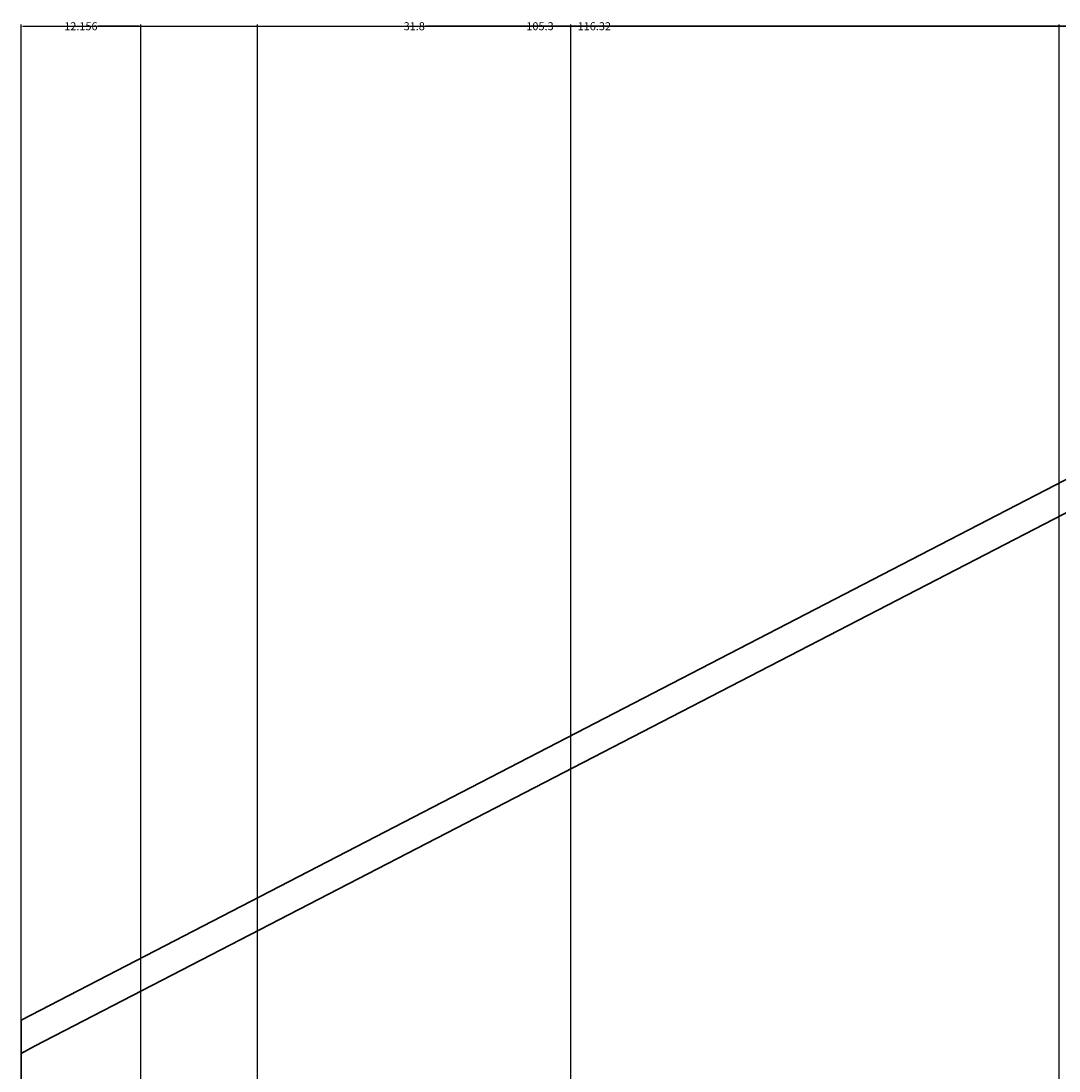
# Model space of a CAD drawing. Units: inches. Extents: x 69 to 650, y -16 to 573.
# Tile 16 of 26: x 100 to 205, y 466 to 573. Entities that reach past the tile are written whole.
import ezdxf

# ---------------------------------------------------------------- set-up
doc = ezdxf.new("R2010")
doc.units = ezdxf.units.IN
doc.header["$MEASUREMENT"] = 0
for name, color, linetype, lineweight in [('A-ANNO-DIMS', 2, 'Continuous', 18), ('A-ROOF', 7, 'Continuous', 35), ('A-WALL', 7, 'Continuous', 35)]:
    doc.layers.add(name, color=color, linetype=linetype, lineweight=lineweight)
doc.styles.get("Standard").update_dxf_attribs({"font": 'arial.ttf'})
doc.dimstyles.get("Standard").update_dxf_attribs({"dimtxt": 0.8125, "dimasz": 0.18, "dimexe": 0.18, "dimexo": 0.0625, "dimgap": 0.09, "dimtad": 0, "dimtih": 1, "dimtoh": 1, "dimdec": 4, "dimzin": 0, "dimdsep": 46, "dimlunit": 4, "dimtxsty": 'Standard', "dimcen": 0.09, "dimadec": 0, "dimazin": 0, "dimtfac": 1, "dimtdec": 4, "dimtofl": 0, "dimtmove": 0, "dimatfit": 3, "dimfxl": 1, "dimtolj": 1, "dimtzin": 0, "dimarcsym": 0})

# ---------------------------------------------------------------- blocks, each defined once
blk = doc.blocks.new('*D19')
at = {"layer": 'A-ANNO-DIMS', "color": 0, "lineweight": -2, "transparency": 16777216}
for p, q in [((99.56, 471.72), (99.56, 572.74)), ((99.74, 572.56), (358.57, 572.56)), ((619.38, 572.56), (360.54, 572.56)), ((619.56, 87.99), (619.56, 572.74))]:
    blk.add_line(p, q, dxfattribs=at)
at = {"layer": 'A-ANNO-DIMS', "color": 0, "transparency": 16777216}
for points in [[(99.74, 572.59), (99.74, 572.53), (99.56, 572.56)], [(619.38, 572.59), (619.38, 572.53), (619.56, 572.56)]]:
    blk.add_solid(points, dxfattribs=at)
at = {"layer": 'Defpoints', "color": 0, "transparency": 16777216}
for p in [(619.56, 572.56), (99.56, 471.66), (619.56, 87.93)]:
    blk.add_point(p, dxfattribs=at)
at = {"layer": 'A-ANNO-DIMS', "color": 0, "transparency": 16777216, "insert": (359.56, 572.56), "char_height": 0.812, "attachment_point": 5}
blk.add_mtext('\\A1;520', dxfattribs=at)
blk = doc.blocks.new('*D49')
at = {"layer": 'A-ANNO-DIMS', "color": 0, "lineweight": -2, "transparency": 16777216}
for p, q in [((99.56, 471.72), (99.56, 572.74)), ((99.74, 572.56), (155.98, 572.56)), ((215.7, 572.56), (159.45, 572.56)), ((215.88, 544.22), (215.88, 572.74))]:
    blk.add_line(p, q, dxfattribs=at)
at = {"layer": 'A-ANNO-DIMS', "color": 0, "transparency": 16777216}
for points in [[(99.74, 572.59), (99.74, 572.53), (99.56, 572.56)], [(215.7, 572.59), (215.7, 572.53), (215.88, 572.56)]]:
    blk.add_solid(points, dxfattribs=at)
at = {"layer": 'Defpoints', "color": 0, "transparency": 16777216}
for p in [(215.88, 572.56), (215.88, 544.16), (99.56, 471.66)]:
    blk.add_point(p, dxfattribs=at)
at = {"layer": 'A-ANNO-DIMS', "color": 0, "transparency": 16777216, "insert": (157.72, 572.56), "char_height": 0.812, "attachment_point": 5}
blk.add_mtext('\\A1;116.32', dxfattribs=at)
blk = doc.blocks.new('*D53')
at = {"layer": 'A-ANNO-DIMS', "color": 0, "lineweight": -2, "transparency": 16777216}
for p, q in [((99.56, 411.99), (99.56, 572.74)), ((99.74, 572.56), (103.9, 572.56)), ((111.53, 572.56), (107.37, 572.56)), ((111.71, 414.48), (111.71, 572.74))]:
    blk.add_line(p, q, dxfattribs=at)
at = {"layer": 'A-ANNO-DIMS', "color": 0, "transparency": 16777216}
for points in [[(99.74, 572.59), (99.74, 572.53), (99.56, 572.56)], [(111.53, 572.59), (111.53, 572.53), (111.71, 572.56)]]:
    blk.add_solid(points, dxfattribs=at)
at = {"layer": 'Defpoints', "color": 0, "transparency": 16777216}
for p in [(111.71, 572.56), (111.71, 414.41), (99.56, 411.93)]:
    blk.add_point(p, dxfattribs=at)
at = {"layer": 'A-ANNO-DIMS', "color": 0, "transparency": 16777216, "insert": (105.63, 572.56), "char_height": 0.812, "attachment_point": 5}
blk.add_mtext('\\A1;12.156', dxfattribs=at)
blk = doc.blocks.new('*D54')
at = {"layer": 'A-ANNO-DIMS', "color": 0, "lineweight": -2, "transparency": 16777216}
for p, q in [((123.55, 432.36), (123.55, 572.74)), ((123.73, 572.56), (138.31, 572.56)), ((155.17, 572.56), (140.6, 572.56)), ((155.35, 432.36), (155.35, 572.74))]:
    blk.add_line(p, q, dxfattribs=at)
at = {"layer": 'A-ANNO-DIMS', "color": 0, "transparency": 16777216}
for points in [[(123.73, 572.59), (123.73, 572.53), (123.55, 572.56)], [(155.17, 572.59), (155.17, 572.53), (155.35, 572.56)]]:
    blk.add_solid(points, dxfattribs=at)
at = {"layer": 'Defpoints', "color": 0, "transparency": 16777216}
for p in [(155.35, 572.56), (123.55, 432.3), (155.35, 432.3)]:
    blk.add_point(p, dxfattribs=at)
at = {"layer": 'A-ANNO-DIMS', "color": 0, "transparency": 16777216, "insert": (139.45, 572.56), "char_height": 0.812, "attachment_point": 5}
blk.add_mtext('\\A1;31.8', dxfattribs=at)
blk = doc.blocks.new('*D61')
at = {"layer": 'A-ANNO-DIMS', "color": 0, "lineweight": -2, "transparency": 16777216}
for p, q in [((99.56, 471.72), (99.56, 572.74)), ((99.74, 572.56), (150.79, 572.56)), ((204.69, 572.56), (153.63, 572.56)), ((204.87, 452.8), (204.87, 572.74))]:
    blk.add_line(p, q, dxfattribs=at)
at = {"layer": 'A-ANNO-DIMS', "color": 0, "transparency": 16777216}
for points in [[(99.74, 572.59), (99.74, 572.53), (99.56, 572.56)], [(204.69, 572.59), (204.69, 572.53), (204.87, 572.56)]]:
    blk.add_solid(points, dxfattribs=at)
at = {"layer": 'Defpoints', "color": 0, "transparency": 16777216}
for p in [(204.87, 572.56), (99.56, 471.66), (204.87, 452.74)]:
    blk.add_point(p, dxfattribs=at)
at = {"layer": 'A-ANNO-DIMS', "color": 0, "transparency": 16777216, "insert": (152.21, 572.56), "char_height": 0.812, "attachment_point": 5}
blk.add_mtext('\\A1;105.3', dxfattribs=at)
blk = doc.blocks.new('*D62')
at = {"layer": 'A-ANNO-DIMS', "color": 0, "lineweight": -2, "transparency": 16777216}
for p, q in [((204.87, 452.8), (204.87, 572.74)), ((205.05, 572.56), (356.52, 572.56)), ((510.91, 572.56), (359.44, 572.56)), ((511.09, 451.98), (511.09, 572.74))]:
    blk.add_line(p, q, dxfattribs=at)
at = {"layer": 'A-ANNO-DIMS', "color": 0, "transparency": 16777216}
for points in [[(205.05, 572.59), (205.05, 572.53), (204.87, 572.56)], [(510.91, 572.59), (510.91, 572.53), (511.09, 572.56)]]:
    blk.add_solid(points, dxfattribs=at)
at = {"layer": 'Defpoints', "color": 0, "transparency": 16777216}
for p in [(511.09, 572.56), (204.87, 452.74), (511.09, 451.92)]:
    blk.add_point(p, dxfattribs=at)
at = {"layer": 'A-ANNO-DIMS', "color": 0, "transparency": 16777216, "insert": (357.98, 572.56), "char_height": 0.812, "attachment_point": 5}
blk.add_mtext('\\A1;306.2', dxfattribs=at)

msp = doc.modelspace()

# ---------------------------------------------------------------- linework, layer by layer
at = {"layer": 'A-ROOF'}
for p, q in [((99.556, 471.6595), (218.848, 533.4142)), ((100.9352, 468.9953), (218.848, 530.036)), ((100.9352, 468.9953), (99.556, 468.2814))]:
    msp.add_line(p, q, dxfattribs=at)
at = {"layer": 'A-WALL'}
msp.add_line((99.556, 411.93), (99.556, 471.6595), dxfattribs=at)

# ---------------------------------------------------------------- dimensions: what is measured, and where the dimension line sits
at = {"layer": 'A-ANNO-DIMS'}
for base, p1, p2, override, picture, middle in [((619.555, 572.5573), (99.556, 471.6595), (619.555, 87.93), {"dimdec": 0, "dimlfac": 1, "dimrnd": 0, "dimzin": 0, "dimdsep": 46, "dimlunit": 2}, '*D19', (359.5555, 572.5573)), ((215.8767, 572.5573), (99.556, 471.6595), (215.8767, 544.1573), {"dimdec": 2, "dimlfac": 1, "dimrnd": 0, "dimzin": 0, "dimdsep": 46, "dimlunit": 2}, '*D49', (157.7164, 572.5573)), ((111.7119, 572.5573), (99.556, 411.93), (111.7119, 414.4146), {"dimdec": 3, "dimlfac": 1, "dimrnd": 0, "dimzin": 0, "dimdsep": 46, "dimlunit": 2}, '*D53', (105.634, 572.5573)), ((204.8658, 572.5573), (99.556, 471.6595), (204.8658, 452.7384), {"dimdec": 1, "dimlfac": 1, "dimrnd": 0, "dimzin": 0, "dimdsep": 46, "dimlunit": 2}, '*D61', (152.2109, 572.5573)), ((155.3536, 572.5573), (123.5533, 432.2961), (155.3536, 432.2961), {"dimdec": 1, "dimlfac": 1, "dimrnd": 0, "dimzin": 0, "dimdsep": 46, "dimlunit": 2}, '*D54', (139.4534, 572.5573)), ((511.0913, 572.5573), (204.8658, 452.7384), (511.0913, 451.9213), {"dimdec": 1, "dimlfac": 1, "dimrnd": 0, "dimzin": 0, "dimdsep": 46, "dimlunit": 2}, '*D62', (357.9786, 572.5573))]:
    dim = msp.add_linear_dim(base=base, p1=p1, p2=p2, dimstyle='Standard', override=override, dxfattribs=at)
    dim.commit()
    dim.dimension.update_dxf_attribs({"geometry": picture, "text_midpoint": middle})

doc.saveas('drawing.dxf')
